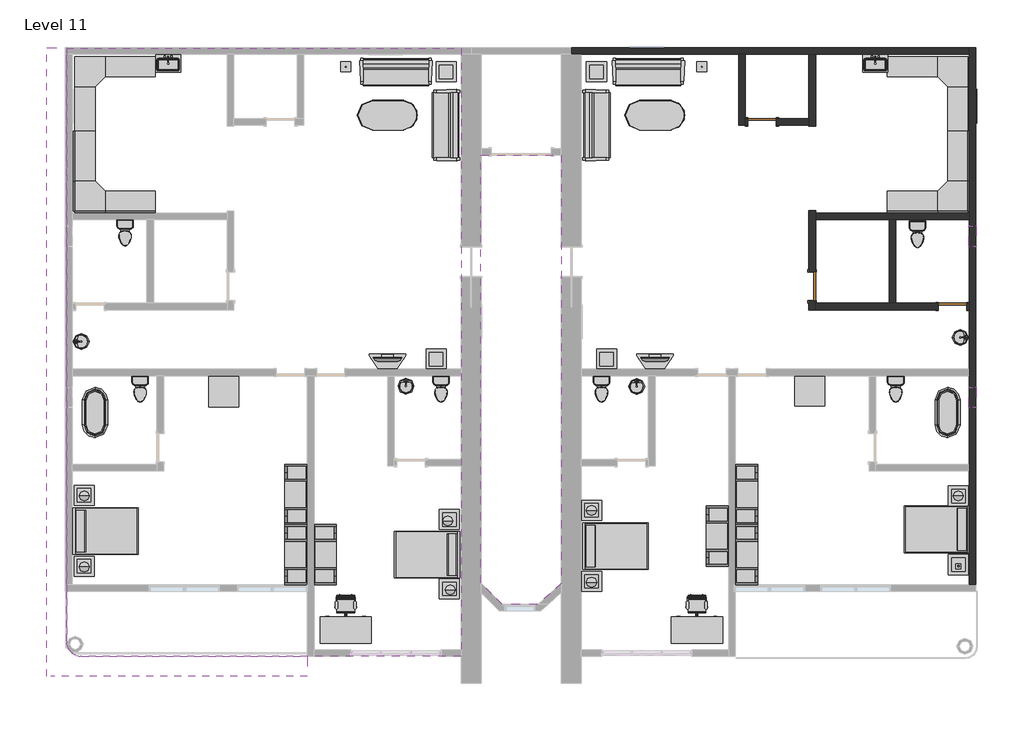
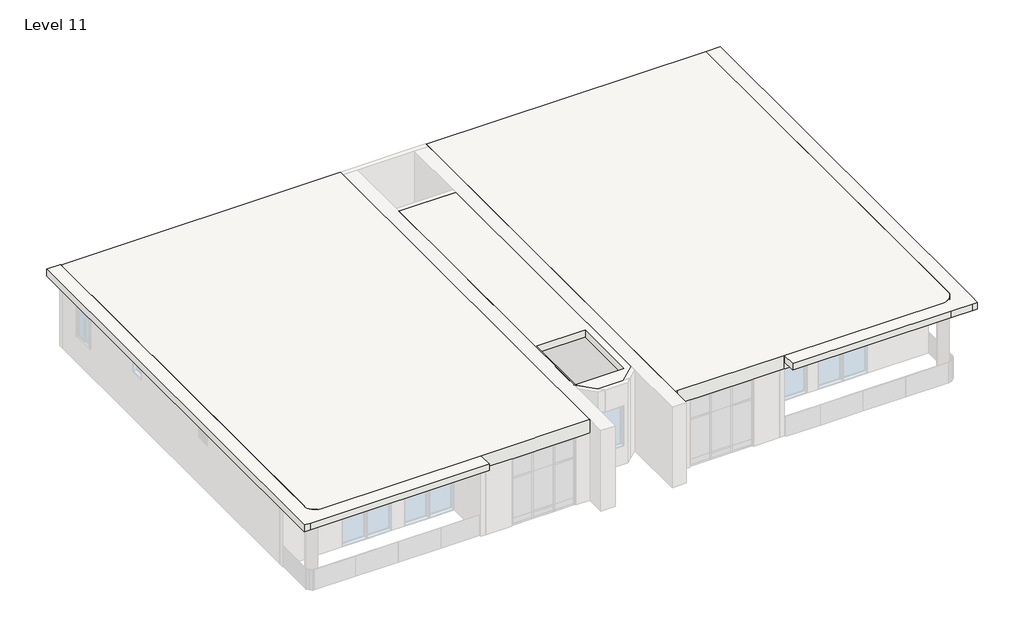
# One storey, part 3 of 3: 42 furniture elements, 14 flow terminals, 10 light fixtures, 9 walls, 3 doors, 3 slabs, 3 windows.
"""IFC4 building model written with IfcOpenShell, lengths in millimetres."""

from ifc_helpers import new_model, si_unit, point, frame, frame_2d, origin, place, context, project, spatial, polyline, circle_curve, trimmed, segment, composite_curve, outline, extrude, faceted_brep, transform, mapped, element, save
from components import door_2703ae13, door_10fd3a06, flow_terminal_38af2918, flow_terminal_d49f872f, toilet_domestic_3d_toilet_domestic_3d_f7549cf7, toilet_domestic_3d_toilet_domestic_3d_183bbd19, flow_terminal_b374fae2, furniture_07436f11, furniture_096e7f55, chair_task_arms_chair_task_arms_fa5a08ef, furniture_072f6425, furniture_cf0b6580, furniture_aff9b2fb, furniture_56245f3a, tv_stand_tv_stand_6ce107e5, furniture_b5c51a22, furniture_2c34a4f9, furniture_4d44e21c, furniture_45e3acac, light_fixture_100w_120v_8564026f, table_lamp_hemispheric_60w_120v_02721d88, window_0038ecf3, window_54100e87

model = new_model("IFC4")

# Units and contexts
model_context = context("Model", 3, world=origin())
ifc_project = project(units=[si_unit("LENGTHUNIT", "METRE", prefix="MILLI")], contexts=[model_context])

# Site, building, storey
site = spatial("IfcSite", under=ifc_project)
building = spatial("IfcBuilding", under=site)
storey = spatial("IfcBuildingStorey", under=building, Name="Level 11", Elevation=36576.0)

# Doors
placement = place(None, origin())
door_shape = door_2703ae13(model_context)
element("IfcDoor", 1, ObjectType="Door-Single-Panel.0001 : 34\" x 80\"", at=placement, inside=storey, context=model_context, shape_type="MappedRepresentation", body=[
    mapped(door_shape, transform((2528.3512296, 9464.0758558, 36576.0), x_axis=(-1.0, 0.0, 0.0), y_axis=(0.0, -1.0, 0.0), z_axis=(0.0, 0.0, 1.0))),
])
door_2_shape = door_10fd3a06(model_context)
element("IfcDoor", 2, ObjectType="Door-Single-Panel.0001 : 34\" x 80\"", at=placement, inside=storey, context=model_context, shape_type="MappedRepresentation", body=[
    mapped(door_2_shape, transform((8319.5512296, 3850.6758558, 36576.0), x_axis=(1.0, 0.0, 0.0), y_axis=(0.0, 1.0, 0.0), z_axis=(0.0, 0.0, 1.0))),
])
element("IfcDoor", 3, ObjectType="Door-Single-Panel.0001 : 34\" x 80\"", at=placement, inside=storey, context=model_context, shape_type="MappedRepresentation", body=[
    mapped(door_2_shape, transform((4052.3512296, 4460.2758558, 36576.0), x_axis=(0.0, -1.0, 0.0), y_axis=(1.0, 0.0, 0.0), z_axis=(0.0, 0.0, 1.0))),
])

# Flow terminals
flow_terminal_shape = flow_terminal_38af2918(model_context)
element("IfcFlowTerminal", 4, ObjectType="Sink Kitchen-Single : 30\" x 21\"", at=placement, inside=storey, context=model_context, shape_type="MappedRepresentation", body=[
    mapped(flow_terminal_shape, transform((-15534.038011, 11239.7304546, 36576.0), x_axis=(1.0, 0.0, 0.0), y_axis=(0.0, 1.0, 0.0), z_axis=(0.0, 0.0, 1.0))),
])
element("IfcFlowTerminal", 5, ObjectType="Sink Kitchen-Single : 30\" x 21\"", at=placement, inside=storey, context=model_context, shape_type="MappedRepresentation", body=[
    mapped(flow_terminal_shape, transform((5954.361989, 11239.7304546, 36576.0), x_axis=(1.0, 0.0, 0.0), y_axis=(0.0, 1.0, 0.0), z_axis=(0.0, 0.0, 1.0))),
])
flow_terminal_2_shape = flow_terminal_d49f872f(model_context)
element("IfcFlowTerminal", 6, ObjectType="Sink Vanity-Round : 19\" x 19\"", at=placement, inside=storey, context=model_context, shape_type="MappedRepresentation", body=[
    mapped(flow_terminal_2_shape, transform((-18078.2570794, 2687.2241152, 36576.0), x_axis=(0.0, 1.0, 0.0), y_axis=(-1.0, 0.0, 0.0), z_axis=(0.0, 0.0, 1.0))),
])
element("IfcFlowTerminal", 7, ObjectType="Sink Vanity-Round : 19\" x 19\"", at=placement, inside=storey, context=model_context, shape_type="MappedRepresentation", body=[
    mapped(flow_terminal_2_shape, transform((8468.5749463, 3007.5275963, 36576.0), x_axis=(0.0, -1.0, 0.0), y_axis=(1.0, 0.0, 0.0), z_axis=(0.0, 0.0, 1.0))),
])
element("IfcFlowTerminal", 8, ObjectType="Sink Vanity-Round : 19\" x 19\"", at=placement, inside=storey, context=model_context, shape_type="MappedRepresentation", body=[
    mapped(flow_terminal_2_shape, transform((-8388.700511, 1341.8921141, 36576.0), x_axis=(1.0, 0.0, 0.0), y_axis=(0.0, 1.0, 0.0), z_axis=(0.0, 0.0, 1.0))),
])
element("IfcFlowTerminal", 9, ObjectType="Sink Vanity-Round : 19\" x 19\"", at=placement, inside=storey, context=model_context, shape_type="MappedRepresentation", body=[
    mapped(flow_terminal_2_shape, transform((-1378.300511, 1331.0855344, 36576.0), x_axis=(1.0, 0.0, 0.0), y_axis=(0.0, 1.0, 0.0), z_axis=(0.0, 0.0, 1.0))),
])
toilet_domestic_3d_toilet_domestic_3d_shape = toilet_domestic_3d_toilet_domestic_3d_f7549cf7(model_context)
toilet_domestic_3d_toilet_domestic_3d_2_shape = toilet_domestic_3d_toilet_domestic_3d_183bbd19(model_context)
element("IfcFlowTerminal", 10, ObjectType="Toilet-Domestic-3D : Toilet-Domestic-3D", at=placement, inside=storey, context=model_context, shape_type="MappedRepresentation", body=[
    mapped(toilet_domestic_3d_toilet_domestic_3d_shape, transform((6592.3512296, 1247.7798284, 36576.0), x_axis=(1.0, 0.0, 0.0), y_axis=(0.0, 1.0, 0.0), z_axis=(0.0, 0.0, 1.0))),
    mapped(toilet_domestic_3d_toilet_domestic_3d_2_shape, transform((6592.3512296, 1247.7798284, 36576.0), x_axis=(1.0, 0.0, 0.0), y_axis=(0.0, 1.0, 0.0), z_axis=(0.0, 0.0, 1.0))),
])
element("IfcFlowTerminal", 11, ObjectType="Toilet-Domestic-3D : Toilet-Domestic-3D", at=placement, inside=storey, context=model_context, shape_type="MappedRepresentation", body=[
    mapped(toilet_domestic_3d_toilet_domestic_3d_shape, transform((-2348.4487704, 1247.7798284, 36576.0), x_axis=(1.0, 0.0, 0.0), y_axis=(0.0, 1.0, 0.0), z_axis=(0.0, 0.0, 1.0))),
    mapped(toilet_domestic_3d_toilet_domestic_3d_2_shape, transform((-2348.4487704, 1247.7798284, 36576.0), x_axis=(1.0, 0.0, 0.0), y_axis=(0.0, 1.0, 0.0), z_axis=(0.0, 0.0, 1.0))),
])
element("IfcFlowTerminal", 12, ObjectType="Toilet-Domestic-3D : Toilet-Domestic-3D", at=placement, inside=storey, context=model_context, shape_type="MappedRepresentation", body=[
    mapped(toilet_domestic_3d_toilet_domestic_3d_shape, transform((-16369.2487704, 1247.7798284, 36576.0), x_axis=(1.0, 0.0, 0.0), y_axis=(0.0, 1.0, 0.0), z_axis=(0.0, 0.0, 1.0))),
    mapped(toilet_domestic_3d_toilet_domestic_3d_2_shape, transform((-16369.2487704, 1247.7798284, 36576.0), x_axis=(1.0, 0.0, 0.0), y_axis=(0.0, 1.0, 0.0), z_axis=(0.0, 0.0, 1.0))),
])
element("IfcFlowTerminal", 13, ObjectType="Toilet-Domestic-3D : Toilet-Domestic-3D", at=placement, inside=storey, context=model_context, shape_type="MappedRepresentation", body=[
    mapped(toilet_domestic_3d_toilet_domestic_3d_shape, transform((-16826.4487704, 5997.5798284, 36576.0), x_axis=(1.0, 0.0, 0.0), y_axis=(0.0, 1.0, 0.0), z_axis=(0.0, 0.0, 1.0))),
    mapped(toilet_domestic_3d_toilet_domestic_3d_2_shape, transform((-16826.4487704, 5997.5798284, 36576.0), x_axis=(1.0, 0.0, 0.0), y_axis=(0.0, 1.0, 0.0), z_axis=(0.0, 0.0, 1.0))),
])
element("IfcFlowTerminal", 14, ObjectType="Toilet-Domestic-3D : Toilet-Domestic-3D", at=placement, inside=storey, context=model_context, shape_type="MappedRepresentation", body=[
    mapped(toilet_domestic_3d_toilet_domestic_3d_shape, transform((7252.7512296, 5946.7798284, 36576.0), x_axis=(1.0, 0.0, 0.0), y_axis=(0.0, 1.0, 0.0), z_axis=(0.0, 0.0, 1.0))),
    mapped(toilet_domestic_3d_toilet_domestic_3d_2_shape, transform((7252.7512296, 5946.7798284, 36576.0), x_axis=(1.0, 0.0, 0.0), y_axis=(0.0, 1.0, 0.0), z_axis=(0.0, 0.0, 1.0))),
])
element("IfcFlowTerminal", 15, ObjectType="Toilet-Domestic-3D : Toilet-Domestic-3D", at=placement, inside=storey, context=model_context, shape_type="MappedRepresentation", body=[
    mapped(toilet_domestic_3d_toilet_domestic_3d_shape, transform((-7225.2487704, 1247.7798284, 36576.0), x_axis=(1.0, 0.0, 0.0), y_axis=(0.0, 1.0, 0.0), z_axis=(0.0, 0.0, 1.0))),
    mapped(toilet_domestic_3d_toilet_domestic_3d_2_shape, transform((-7225.2487704, 1247.7798284, 36576.0), x_axis=(1.0, 0.0, 0.0), y_axis=(0.0, 1.0, 0.0), z_axis=(0.0, 0.0, 1.0))),
])
flow_terminal_3_shape = flow_terminal_b374fae2(model_context)
element("IfcFlowTerminal", 16, ObjectType="Tub-Free Standing-3D : 30\" x 60\"", at=placement, inside=storey, context=model_context, shape_type="MappedRepresentation", body=[
    mapped(flow_terminal_3_shape, transform((-17740.8487704, 624.8758558, 36576.0), x_axis=(1.0, 0.0, 0.0), y_axis=(0.0, 1.0, 0.0), z_axis=(0.0, 0.0, 1.0))),
])
element("IfcFlowTerminal", 17, ObjectType="Tub-Free Standing-3D : 30\" x 60\"", at=placement, inside=storey, context=model_context, shape_type="MappedRepresentation", body=[
    mapped(flow_terminal_3_shape, transform((8167.1512296, 624.8758558, 36576.0), x_axis=(1.0, 0.0, 0.0), y_axis=(0.0, 1.0, 0.0), z_axis=(0.0, 0.0, 1.0))),
])

# Furniture
furniture_shape = furniture_07436f11(model_context)
element("IfcFurniture", 18, ObjectType="96\" x 96\"", at=placement, inside=storey, context=model_context, shape_type="MappedRepresentation", body=[
    mapped(furniture_shape, transform((-18269.5170182, 11991.0988634, 36576.0), x_axis=(1.0, 0.0, 0.0), y_axis=(0.0, 1.0, 0.0), z_axis=(0.0, 0.0, 1.0))),
])
element("IfcFurniture", 19, ObjectType="96\" x 96\"", at=placement, inside=storey, context=model_context, shape_type="MappedRepresentation", body=[
    mapped(furniture_shape, transform((9322.5742372, 11364.3441035, 36576.0), x_axis=(0.0, -1.0, 0.0), y_axis=(1.0, 0.0, 0.0), z_axis=(0.0, 0.0, 1.0))),
])
furniture_2_shape = furniture_096e7f55(model_context)
element("IfcFurniture", 20, ObjectType="Bed-Shaker : Double 56\" x 78\"", at=placement, inside=storey, context=model_context, shape_type="MappedRepresentation", body=[
    mapped(furniture_2_shape, transform((-18401.2487704, -2962.8741442, 36576.0), x_axis=(0.0, 1.0, 0.0), y_axis=(-1.0, 0.0, 0.0), z_axis=(0.0, 0.0, 1.0))),
])
element("IfcFurniture", 21, ObjectType="Bed-Shaker : Double 56\" x 78\"", at=placement, inside=storey, context=model_context, shape_type="MappedRepresentation", body=[
    mapped(furniture_2_shape, transform((-6666.4487704, -3712.1741442, 36576.0), x_axis=(0.0, -1.0, 0.0), y_axis=(1.0, 0.0, 0.0), z_axis=(0.0, 0.0, 1.0))),
])
element("IfcFurniture", 22, ObjectType="Bed-Shaker : Double 56\" x 78\"", at=placement, inside=storey, context=model_context, shape_type="MappedRepresentation", body=[
    mapped(furniture_2_shape, transform((-2907.2487704, -3420.0741442, 36576.0), x_axis=(0.0, 1.0, 0.0), y_axis=(-1.0, 0.0, 0.0), z_axis=(0.0, 0.0, 1.0))),
])
element("IfcFurniture", 23, ObjectType="Bed-Shaker : Double 56\" x 78\"", at=placement, inside=storey, context=model_context, shape_type="MappedRepresentation", body=[
    mapped(furniture_2_shape, transform((8827.5512296, -2950.1741442, 36576.0), x_axis=(0.0, -1.0, 0.0), y_axis=(1.0, 0.0, 0.0), z_axis=(0.0, 0.0, 1.0))),
])
chair_task_arms_chair_task_arms_shape = chair_task_arms_chair_task_arms_fa5a08ef(model_context)
element("IfcFurniture", 24, ObjectType="Chair-Task Arms : Chair-Task Arms", at=placement, inside=storey, context=model_context, shape_type="MappedRepresentation", body=[
    mapped(chair_task_arms_chair_task_arms_shape, transform((688.1420493, -5184.3566833, 36576.0), x_axis=(-1.0, 0.0, 0.0), y_axis=(0.0, -1.0, 0.0), z_axis=(0.0, 0.0, 1.0))),
])
element("IfcFurniture", 25, ObjectType="Chair-Task Arms : Chair-Task Arms", at=placement, inside=storey, context=model_context, shape_type="MappedRepresentation", body=[
    mapped(chair_task_arms_chair_task_arms_shape, transform((-9979.8579507, -5184.3566833, 36576.0), x_axis=(-1.0, 0.0, 0.0), y_axis=(0.0, -1.0, 0.0), z_axis=(0.0, 0.0, 1.0))),
])
furniture_3_shape = furniture_072f6425(model_context)
element("IfcFurniture", 26, ObjectType="Desk : 60\" x 30\"", at=placement, inside=storey, context=model_context, shape_type="MappedRepresentation", body=[
    mapped(furniture_3_shape, transform((-10882.8487704, -6371.702585, 36576.0), x_axis=(1.0, 0.0, 0.0), y_axis=(0.0, 1.0, 0.0), z_axis=(0.0, 0.0, 1.0))),
])
element("IfcFurniture", 27, ObjectType="Desk : 60\" x 30\"", at=placement, inside=storey, context=model_context, shape_type="MappedRepresentation", body=[
    mapped(furniture_3_shape, transform((-214.8487704, -6371.702585, 36576.0), x_axis=(1.0, 0.0, 0.0), y_axis=(0.0, 1.0, 0.0), z_axis=(0.0, 0.0, 1.0))),
])
furniture_4_shape = furniture_cf0b6580(model_context)
element("IfcFurniture", 28, ObjectType="Entertainment Center : 72\" x 72\" x 24\"", at=placement, inside=storey, context=model_context, shape_type="MappedRepresentation", body=[
    mapped(furniture_4_shape, transform((1613.9512296, -3134.3241442, 36576.0), x_axis=(0.0, -1.0, 0.0), y_axis=(1.0, 0.0, 0.0), z_axis=(0.0, 0.0, 1.0))),
])
element("IfcFurniture", 29, ObjectType="Entertainment Center : 72\" x 72\" x 24\"", at=placement, inside=storey, context=model_context, shape_type="MappedRepresentation", body=[
    mapped(furniture_4_shape, transform((1613.9512296, -3693.1241442, 36576.0), x_axis=(0.0, 1.0, 0.0), y_axis=(-1.0, 0.0, 0.0), z_axis=(0.0, 0.0, 1.0))),
])
element("IfcFurniture", 30, ObjectType="Entertainment Center : 72\" x 72\" x 24\"", at=placement, inside=storey, context=model_context, shape_type="MappedRepresentation", body=[
    mapped(furniture_4_shape, transform((1613.9512296, -1864.3241442, 36576.0), x_axis=(0.0, 1.0, 0.0), y_axis=(-1.0, 0.0, 0.0), z_axis=(0.0, 0.0, 1.0))),
])
element("IfcFurniture", 31, ObjectType="Entertainment Center : 72\" x 72\" x 24\"", at=placement, inside=storey, context=model_context, shape_type="MappedRepresentation", body=[
    mapped(furniture_4_shape, transform((-11187.6487704, -3693.1241442, 36576.0), x_axis=(0.0, -1.0, 0.0), y_axis=(1.0, 0.0, 0.0), z_axis=(0.0, 0.0, 1.0))),
])
element("IfcFurniture", 32, ObjectType="Entertainment Center : 72\" x 72\" x 24\"", at=placement, inside=storey, context=model_context, shape_type="MappedRepresentation", body=[
    mapped(furniture_4_shape, transform((-11187.6487704, -1864.3241442, 36576.0), x_axis=(0.0, -1.0, 0.0), y_axis=(1.0, 0.0, 0.0), z_axis=(0.0, 0.0, 1.0))),
])
element("IfcFurniture", 33, ObjectType="Entertainment Center : 72\" x 72\" x 24\"", at=placement, inside=storey, context=model_context, shape_type="MappedRepresentation", body=[
    mapped(furniture_4_shape, transform((-11187.6487704, -3693.1241442, 36576.0), x_axis=(0.0, 1.0, 0.0), y_axis=(-1.0, 0.0, 0.0), z_axis=(0.0, 0.0, 1.0))),
])
furniture_5_shape = furniture_aff9b2fb(model_context)
element("IfcFurniture", 34, ObjectType="Sofa-Pensi : 84\"", at=placement, inside=storey, context=model_context, shape_type="MappedRepresentation", body=[
    mapped(furniture_5_shape, transform((-8875.4550204, 10710.9660197, 36576.0), x_axis=(1.0, 0.0, 0.0), y_axis=(0.0, 1.0, 0.0), z_axis=(0.0, 0.0, 1.0))),
])
element("IfcFurniture", 35, ObjectType="Sofa-Pensi : 84\"", at=placement, inside=storey, context=model_context, shape_type="MappedRepresentation", body=[
    mapped(furniture_5_shape, transform((-7349.9586065, 9641.0821058, 36576.0), x_axis=(0.0, -1.0, 0.0), y_axis=(1.0, 0.0, 0.0), z_axis=(0.0, 0.0, 1.0))),
])
element("IfcFurniture", 36, ObjectType="Sofa-Pensi : 84\"", at=placement, inside=storey, context=model_context, shape_type="MappedRepresentation", body=[
    mapped(furniture_5_shape, transform((-2223.7389343, 9083.8696058, 36576.0), x_axis=(0.0, 1.0, 0.0), y_axis=(-1.0, 0.0, 0.0), z_axis=(0.0, 0.0, 1.0))),
])
element("IfcFurniture", 37, ObjectType="Sofa-Pensi : 84\"", at=placement, inside=storey, context=model_context, shape_type="MappedRepresentation", body=[
    mapped(furniture_5_shape, transform((-1204.6550204, 10710.9660197, 36576.0), x_axis=(1.0, 0.0, 0.0), y_axis=(0.0, 1.0, 0.0), z_axis=(0.0, 0.0, 1.0))),
])
furniture_6_shape = furniture_56245f3a(model_context)
element("IfcFurniture", 38, ObjectType="TV - Flat Screen : 32\"", at=placement, inside=storey, context=model_context, shape_type="MappedRepresentation", body=[
    mapped(furniture_6_shape, transform((-8854.7932846, 2232.8144794, 37490.4), x_axis=(-1.0, 0.0, 0.0), y_axis=(0.0, -1.0, 0.0), z_axis=(0.0, 0.0, 1.0))),
])
element("IfcFurniture", 39, ObjectType="TV - Flat Screen : 32\"", at=placement, inside=storey, context=model_context, shape_type="MappedRepresentation", body=[
    mapped(furniture_6_shape, transform((-726.7932846, 2232.8144794, 37490.4), x_axis=(-1.0, 0.0, 0.0), y_axis=(0.0, -1.0, 0.0), z_axis=(0.0, 0.0, 1.0))),
])
tv_stand_tv_stand_shape = tv_stand_tv_stand_6ce107e5(model_context)
element("IfcFurniture", 40, ObjectType="TV Stand : TV Stand", at=placement, inside=storey, context=model_context, shape_type="MappedRepresentation", body=[
    mapped(tv_stand_tv_stand_shape, transform((-8725.6607683, 1945.6758558, 36576.0), x_axis=(-1.0, 0.0, 0.0), y_axis=(0.0, -1.0, 0.0), z_axis=(0.0, 0.0, 1.0))),
])
element("IfcFurniture", 41, ObjectType="TV Stand : TV Stand", at=placement, inside=storey, context=model_context, shape_type="MappedRepresentation", body=[
    mapped(tv_stand_tv_stand_shape, transform((-597.6607683, 1945.6758558, 36576.0), x_axis=(-1.0, 0.0, 0.0), y_axis=(0.0, -1.0, 0.0), z_axis=(0.0, 0.0, 1.0))),
])
furniture_7_shape = furniture_b5c51a22(model_context)
element("IfcFurniture", 42, ObjectType="Table-Coffee : 24\" x 24\" x 24\"", at=placement, inside=storey, context=model_context, shape_type="MappedRepresentation", body=[
    mapped(furniture_7_shape, transform((-7091.1145371, 10892.864778, 36576.0), x_axis=(1.0, 0.0, 0.0), y_axis=(0.0, 1.0, 0.0), z_axis=(0.0, 0.0, 1.0))),
])
element("IfcFurniture", 43, ObjectType="Table-Coffee : 24\" x 24\" x 24\"", at=placement, inside=storey, context=model_context, shape_type="MappedRepresentation", body=[
    mapped(furniture_7_shape, transform((-2519.1145371, 10892.864778, 36576.0), x_axis=(1.0, 0.0, 0.0), y_axis=(0.0, 1.0, 0.0), z_axis=(0.0, 0.0, 1.0))),
])
element("IfcFurniture", 44, ObjectType="Table-Coffee : 24\" x 24\" x 24\"", at=placement, inside=storey, context=model_context, shape_type="MappedRepresentation", body=[
    mapped(furniture_7_shape, transform((-7395.9145371, 2155.264778, 36576.0), x_axis=(1.0, 0.0, 0.0), y_axis=(0.0, 1.0, 0.0), z_axis=(0.0, 0.0, 1.0))),
])
element("IfcFurniture", 45, ObjectType="Table-Coffee : 24\" x 24\" x 24\"", at=placement, inside=storey, context=model_context, shape_type="MappedRepresentation", body=[
    mapped(furniture_7_shape, transform((-2214.3145371, 2155.264778, 36576.0), x_axis=(1.0, 0.0, 0.0), y_axis=(0.0, 1.0, 0.0), z_axis=(0.0, 0.0, 1.0))),
])
element("IfcFurniture", 46, ObjectType="Table-Coffee : 24\" x 24\" x 24\"", at=placement, inside=storey, context=model_context, shape_type="MappedRepresentation", body=[
    mapped(furniture_7_shape, transform((-2671.5145371, -4601.135222, 36576.0), x_axis=(1.0, 0.0, 0.0), y_axis=(0.0, 1.0, 0.0), z_axis=(0.0, 0.0, 1.0))),
])
element("IfcFurniture", 47, ObjectType="Table-Coffee : 24\" x 24\" x 24\"", at=placement, inside=storey, context=model_context, shape_type="MappedRepresentation", body=[
    mapped(furniture_7_shape, transform((-18089.3145371, -4143.935222, 36576.0), x_axis=(1.0, 0.0, 0.0), y_axis=(0.0, 1.0, 0.0), z_axis=(0.0, 0.0, 1.0))),
])
element("IfcFurniture", 48, ObjectType="Table-Coffee : 24\" x 24\" x 24\"", at=placement, inside=storey, context=model_context, shape_type="MappedRepresentation", body=[
    mapped(furniture_7_shape, transform((-18089.3145371, -1984.935222, 36576.0), x_axis=(1.0, 0.0, 0.0), y_axis=(0.0, 1.0, 0.0), z_axis=(0.0, 0.0, 1.0))),
])
element("IfcFurniture", 49, ObjectType="Table-Coffee : 24\" x 24\" x 24\"", at=placement, inside=storey, context=model_context, shape_type="MappedRepresentation", body=[
    mapped(furniture_7_shape, transform((-2671.5145371, -2442.135222, 36576.0), x_axis=(1.0, 0.0, 0.0), y_axis=(0.0, 1.0, 0.0), z_axis=(0.0, 0.0, 1.0))),
])
element("IfcFurniture", 50, ObjectType="Table-Coffee : 24\" x 24\" x 24\"", at=placement, inside=storey, context=model_context, shape_type="MappedRepresentation", body=[
    mapped(furniture_7_shape, transform((8479.0854629, -4093.135222, 36576.0), x_axis=(1.0, 0.0, 0.0), y_axis=(0.0, 1.0, 0.0), z_axis=(0.0, 0.0, 1.0))),
])
element("IfcFurniture", 51, ObjectType="Table-Coffee : 24\" x 24\" x 24\"", at=placement, inside=storey, context=model_context, shape_type="MappedRepresentation", body=[
    mapped(furniture_7_shape, transform((8479.0854629, -2010.335222, 36576.0), x_axis=(1.0, 0.0, 0.0), y_axis=(0.0, 1.0, 0.0), z_axis=(0.0, 0.0, 1.0))),
])
element("IfcFurniture", 52, ObjectType="Table-Coffee : 24\" x 24\" x 24\"", at=placement, inside=storey, context=model_context, shape_type="MappedRepresentation", body=[
    mapped(furniture_7_shape, transform((-6989.5145371, -4832.0414601, 36576.0), x_axis=(1.0, 0.0, 0.0), y_axis=(0.0, 1.0, 0.0), z_axis=(0.0, 0.0, 1.0))),
])
element("IfcFurniture", 53, ObjectType="Table-Coffee : 24\" x 24\" x 24\"", at=placement, inside=storey, context=model_context, shape_type="MappedRepresentation", body=[
    mapped(furniture_7_shape, transform((-6989.5145371, -2723.8414601, 36576.0), x_axis=(1.0, 0.0, 0.0), y_axis=(0.0, 1.0, 0.0), z_axis=(0.0, 0.0, 1.0))),
])
furniture_8_shape = furniture_2c34a4f9(model_context)
element("IfcFurniture", 54, ObjectType="Table-Dining Oval : 36\" x 72\"", at=placement, inside=storey, context=model_context, shape_type="MappedRepresentation", body=[
    mapped(furniture_8_shape, transform((-8449.0290983, 10025.3742164, 36576.0), x_axis=(1.0, 0.0, 0.0), y_axis=(0.0, 1.0, 0.0), z_axis=(0.0, 0.0, 1.0))),
])
element("IfcFurniture", 55, ObjectType="Table-Dining Oval : 36\" x 72\"", at=placement, inside=storey, context=model_context, shape_type="MappedRepresentation", body=[
    mapped(furniture_8_shape, transform((-321.0290983, 10025.3742164, 36576.0), x_axis=(1.0, 0.0, 0.0), y_axis=(0.0, 1.0, 0.0), z_axis=(0.0, 0.0, 1.0))),
])
furniture_9_shape = furniture_4d44e21c(model_context)
element("IfcFurniture", 56, ObjectType="Table-Rectangular : 36\" x 36\"", at=placement, inside=storey, context=model_context, shape_type="MappedRepresentation", body=[
    mapped(furniture_9_shape, transform((-13829.2487704, 1259.8758558, 36576.0), x_axis=(1.0, 0.0, 0.0), y_axis=(0.0, 1.0, 0.0), z_axis=(0.0, 0.0, 1.0))),
])
element("IfcFurniture", 57, ObjectType="Table-Rectangular : 36\" x 36\"", at=placement, inside=storey, context=model_context, shape_type="MappedRepresentation", body=[
    mapped(furniture_9_shape, transform((3976.1512296, 1285.2758558, 36576.0), x_axis=(1.0, 0.0, 0.0), y_axis=(0.0, 1.0, 0.0), z_axis=(0.0, 0.0, 1.0))),
])
furniture_10_shape = furniture_45e3acac(model_context)
element("IfcFurniture", 58, ObjectType="Work Station Cubicle : 96\" x 96\"", at=placement, inside=storey, context=model_context, shape_type="MappedRepresentation", body=[
    mapped(furniture_10_shape, transform((-18896.271778, 6827.207608, 36576.0), x_axis=(0.0, 1.0, 0.0), y_axis=(-1.0, 0.0, 0.0), z_axis=(0.0, 0.0, 1.0))),
])
element("IfcFurniture", 59, ObjectType="Work Station Cubicle : 96\" x 96\"", at=placement, inside=storey, context=model_context, shape_type="MappedRepresentation", body=[
    mapped(furniture_10_shape, transform((8695.8194774, 6200.4528481, 36576.0), x_axis=(-1.0, 0.0, 0.0), y_axis=(0.0, -1.0, 0.0), z_axis=(0.0, 0.0, 1.0))),
])

# Light fixtures
light_fixture_100w_120v_shape = light_fixture_100w_120v_8564026f(model_context)
element("IfcLightFixture", 60, ObjectType="100W - 120V", at=placement, inside=storey, context=model_context, shape_type="MappedRepresentation", body=[
    mapped(light_fixture_100w_120v_shape, transform((-10120.8487704, 11140.4758558, 36576.0), x_axis=(1.0, 0.0, 0.0), y_axis=(0.0, 1.0, 0.0), z_axis=(0.0, 0.0, 1.0))),
])
element("IfcLightFixture", 61, ObjectType="100W - 120V", at=placement, inside=storey, context=model_context, shape_type="MappedRepresentation", body=[
    mapped(light_fixture_100w_120v_shape, transform((699.5512296, 11140.4758558, 36576.0), x_axis=(1.0, 0.0, 0.0), y_axis=(0.0, 1.0, 0.0), z_axis=(0.0, 0.0, 1.0))),
])
table_lamp_hemispheric_60w_120v_shape = table_lamp_hemispheric_60w_120v_02721d88(model_context)
element("IfcLightFixture", 62, ObjectType="Table Lamp - Hemispheric : 60W - 120V", at=placement, inside=storey, context=model_context, shape_type="MappedRepresentation", body=[
    mapped(table_lamp_hemispheric_60w_120v_shape, transform((-18071.0487704, -1915.1241442, 37185.6), x_axis=(1.0, 0.0, 0.0), y_axis=(0.0, 1.0, 0.0), z_axis=(0.0, 0.0, 1.0))),
])
element("IfcLightFixture", 63, ObjectType="Table Lamp - Hemispheric : 60W - 120V", at=placement, inside=storey, context=model_context, shape_type="MappedRepresentation", body=[
    mapped(table_lamp_hemispheric_60w_120v_shape, transform((-7022.0487704, -2666.7303823, 37185.6), x_axis=(1.0, 0.0, 0.0), y_axis=(0.0, 1.0, 0.0), z_axis=(0.0, 0.0, 1.0))),
])
element("IfcLightFixture", 64, ObjectType="Table Lamp - Hemispheric : 60W - 120V", at=placement, inside=storey, context=model_context, shape_type="MappedRepresentation", body=[
    mapped(table_lamp_hemispheric_60w_120v_shape, transform((-2653.2487704, -2346.9241442, 37185.6), x_axis=(1.0, 0.0, 0.0), y_axis=(0.0, 1.0, 0.0), z_axis=(0.0, 0.0, 1.0))),
])
element("IfcLightFixture", 65, ObjectType="Table Lamp - Hemispheric : 60W - 120V", at=placement, inside=storey, context=model_context, shape_type="MappedRepresentation", body=[
    mapped(table_lamp_hemispheric_60w_120v_shape, transform((8497.3512296, -4048.7241442, 37490.4), x_axis=(1.0, 0.0, 0.0), y_axis=(0.0, 1.0, 0.0), z_axis=(0.0, 0.0, 1.0))),
])
element("IfcLightFixture", 66, ObjectType="Table Lamp - Hemispheric : 60W - 120V", at=placement, inside=storey, context=model_context, shape_type="MappedRepresentation", body=[
    mapped(table_lamp_hemispheric_60w_120v_shape, transform((8497.3512296, -1915.1241442, 37185.6), x_axis=(1.0, 0.0, 0.0), y_axis=(0.0, 1.0, 0.0), z_axis=(0.0, 0.0, 1.0))),
])
element("IfcLightFixture", 67, ObjectType="Table Lamp - Hemispheric : 60W - 120V", at=placement, inside=storey, context=model_context, shape_type="MappedRepresentation", body=[
    mapped(table_lamp_hemispheric_60w_120v_shape, transform((-2653.2487704, -4531.3241442, 37185.6), x_axis=(1.0, 0.0, 0.0), y_axis=(0.0, 1.0, 0.0), z_axis=(0.0, 0.0, 1.0))),
])
element("IfcLightFixture", 68, ObjectType="Table Lamp - Hemispheric : 60W - 120V", at=placement, inside=storey, context=model_context, shape_type="MappedRepresentation", body=[
    mapped(table_lamp_hemispheric_60w_120v_shape, transform((-6945.8487704, -4762.2303823, 37185.6), x_axis=(1.0, 0.0, 0.0), y_axis=(0.0, 1.0, 0.0), z_axis=(0.0, 0.0, 1.0))),
])
element("IfcLightFixture", 69, ObjectType="Table Lamp - Hemispheric : 60W - 120V", at=placement, inside=storey, context=model_context, shape_type="MappedRepresentation", body=[
    mapped(table_lamp_hemispheric_60w_120v_shape, transform((-18071.0487704, -4074.1241442, 37185.6), x_axis=(1.0, 0.0, 0.0), y_axis=(0.0, 1.0, 0.0), z_axis=(0.0, 0.0, 1.0))),
])

# Slabs
element("IfcSlab", 70, ObjectType="Generic - 12\" cream", at=placement, inside=storey, context=model_context, shape_type="SweptSolid", body=[
    extrude(outline(composite_curve([segment(polyline([(-6615.6487704, 11699.2758558), (-6615.6487704, -6791.9241442), (-11289.2487704, -6791.9241442), (-18147.2487704, -6791.9241442)]), True, "CONTINUOUS"), segment(trimmed(circle_curve(frame_2d((-18147.2487704, -6334.7241442)), 457.2), [point((-18147.2487704, -6791.9241442))], [point((-18604.4487704, -6334.7241442))], False, "CARTESIAN"), True, "CONTINUOUS"), segment(polyline([(-18604.4487704, -6334.7241442), (-18604.4487704, 11699.2758558), (-6615.6487704, 11699.2758558)]), True, "CONTINUOUS")], self_intersect=False)), frame((0.0, 0.0, 39624.0), z_axis=(0.0, 0.0, 1.0), x_axis=(1.0, 0.0, 0.0)), (0.0, 0.0, 1.0), 609.6),
    extrude(outline(composite_curve([segment(trimmed(circle_curve(frame_2d((8518.1543381, -6277.3874522)), 514.536692), [point((9030.7512296, -6322.0241442))], [point((8518.1543381, -6791.9241442))], False, "CARTESIAN"), True, "CONTINUOUS"), segment(polyline([(8518.1543381, -6791.9241442), (1715.5512296, -6791.9241442), (-2856.4487704, -6791.9241442), (-2958.0487704, -6791.9241442), (-2958.0487704, 11699.2758558), (9030.7512296, 11699.2758558), (9030.7512296, -6322.0241442)]), True, "CONTINUOUS")], self_intersect=False)), frame((0.0, 0.0, 39624.0), z_axis=(0.0, 0.0, 1.0), x_axis=(1.0, 0.0, 0.0)), (0.0, 0.0, 1.0), 609.6),
])
element("IfcSlab", 71, ObjectType="Generic - 12\" white", at=placement, inside=storey, context=model_context, shape_type="SweptSolid", body=[
    extrude(outline(composite_curve([segment(polyline([(9640.3512296, 11699.2758558), (9640.3512296, -6931.6241442), (9640.3512296, -7401.5241442), (9437.1512296, -7401.5241442), (8518.1543381, -7401.5241442), (1715.5512296, -7401.5241442), (1715.5512296, -6791.9241442), (8518.1543381, -6791.9241442)]), True, "CONTINUOUS"), segment(trimmed(circle_curve(frame_2d((8518.1543381, -6277.3874522)), 514.536692), [point((8518.1543381, -6791.9241442))], [point((9030.7512296, -6322.0241442))], True, "CARTESIAN"), True, "CONTINUOUS"), segment(polyline([(9030.7512296, -6322.0241442), (9030.7512296, 11699.2758558), (9640.3512296, 11699.2758558)]), True, "CONTINUOUS")], self_intersect=False)), frame((0.0, 0.0, 39928.8), z_axis=(0.0, 0.0, 1.0), x_axis=(1.0, 0.0, 0.0)), (0.0, 0.0, 1.0), 304.8),
    extrude(outline(composite_curve([segment(polyline([(-18604.4487704, 11724.6758558), (-18604.4487704, -6334.7241442)]), True, "CONTINUOUS"), segment(trimmed(circle_curve(frame_2d((-18147.2487704, -6334.7241442)), 457.2), [point((-18604.4487704, -6334.7241442))], [point((-18147.2487704, -6791.9241442))], True, "CARTESIAN"), True, "CONTINUOUS"), segment(polyline([(-18147.2487704, -6791.9241442), (-11289.2487704, -6791.9241442), (-11289.2487704, -7401.5241442), (-18960.0487704, -7401.5241442), (-19214.0487704, -7401.5241442), (-19214.0487704, 11724.6758558), (-18604.4487704, 11724.6758558)]), True, "CONTINUOUS")], self_intersect=False)), frame((0.0, 0.0, 39928.8), z_axis=(0.0, 0.0, 1.0), x_axis=(1.0, 0.0, 0.0)), (0.0, 0.0, 1.0), 304.8),
])
element("IfcSlab", 72, ObjectType="Generic - 12\" white", at=placement, inside=storey, context=model_context, shape_type="SweptSolid", body=[
    extrude(outline(polyline([(-3573.9987704, 8448.0758558), (-3573.9987704, -1691.5549149), (-3573.9987704, -4572.9908503), (-4280.7801413, -5203.302585), (-5368.1862318, -5203.302585), (-6012.3987704, -4559.0900463), (-6012.3987704, -1691.5549149), (-6012.3987704, 8448.0758558), (-3573.9987704, 8448.0758558)]), holes=[polyline([(-5940.8822214, -4561.7549149), (-3870.7822214, -4561.7549149), (-3870.7822214, -1691.5549149), (-5940.8822214, -1691.5549149), (-5940.8822214, -4561.7549149)])]), frame((0.0, 0.0, 39928.8), z_axis=(0.0, 0.0, 1.0), x_axis=(1.0, 0.0, 0.0)), (0.0, 0.0, 1.0), 304.8),
])

# Walls
element("IfcWall", 73, ObjectType="Generic - 8\" cream", at=placement, inside=storey, context=model_context, shape_type="Brep", body=[
    faceted_brep([(8827.5512296, 11724.6758558, 36576.0), (8827.5512296, 11521.4758558, 36576.0), (8827.5512296, 6695.4758558, 36576.0), (8827.5512296, 6492.2758558, 36576.0), (8827.5512296, 3952.2758558, 36576.0), (8827.5512296, 3749.0758558, 36576.0), (8827.5512296, 1945.6758558, 36576.0), (8827.5512296, 1742.4758558, 36576.0), (8827.5512296, -949.9241442, 36576.0), (8827.5512296, -1153.1241442, 36576.0), (8827.5512296, -4607.5241442, 36576.0), (8827.5512296, -4607.5241442, 39624.0), (8827.5512296, -1153.1241442, 39624.0), (8827.5512296, -949.9241442, 39624.0), (8827.5512296, 1742.4758558, 39624.0), (8827.5512296, 1945.6758558, 39624.0), (8827.5512296, 3749.0758558, 39624.0), (8827.5512296, 3952.2758558, 39624.0), (8827.5512296, 6492.2758558, 39624.0), (8827.5512296, 6695.4758558, 39624.0), (8827.5512296, 11521.4758558, 39624.0), (8827.5512296, 11724.6758558, 39624.0), (8827.5512296, 10403.8758558, 37795.2), (8827.5512296, 10403.8758558, 39014.4), (8827.5512296, 9489.4758558, 39014.4), (8827.5512296, 9489.4758558, 37795.2), (8827.5512296, 777.2758558, 39319.2), (8827.5512296, 777.2758558, 38709.6), (8827.5512296, 1386.8758558, 38709.6), (8827.5512296, 1386.8758558, 39319.2), (8827.5512296, 6289.0758558, 38709.6), (8827.5512296, 6289.0758558, 39319.2), (8827.5512296, 5679.4758558, 39319.2), (8827.5512296, 5679.4758558, 38709.6), (9030.7512296, -4607.5241442, 36576.0), (9030.7512296, 11724.6758558, 36576.0), (9030.7512296, 11724.6758558, 39624.0), (9030.7512296, -4607.5241442, 39624.0), (9030.7512296, 10403.8758558, 39014.4), (9030.7512296, 10403.8758558, 37795.2), (9030.7512296, 9489.4758558, 37795.2), (9030.7512296, 9489.4758558, 39014.4), (9030.7512296, 777.2758558, 38709.6), (9030.7512296, 777.2758558, 39319.2), (9030.7512296, 1386.8758558, 39319.2), (9030.7512296, 1386.8758558, 38709.6), (9030.7512296, 6289.0758558, 39319.2), (9030.7512296, 6289.0758558, 38709.6), (9030.7512296, 5679.4758558, 38709.6), (9030.7512296, 5679.4758558, 39319.2)], [[[0, 1, 2, 3, 4, 5, 6, 7, 8, 9, 10, 11, 12, 13, 14, 15, 16, 17, 18, 19, 20, 21], [22, 23, 24, 25], [26, 27, 28, 29], [30, 31, 32, 33]], [[34, 35, 36, 37], [38, 39, 40, 41], [42, 43, 44, 45], [46, 47, 48, 49]], [[10, 9, 8, 7, 6, 5, 4, 3, 2, 1, 0, 35, 34]], [[21, 20, 19, 18, 17, 16, 15, 14, 13, 12, 11, 37, 36]], [[0, 21, 36, 35]], [[11, 10, 34, 37]], [[39, 38, 23, 22]], [[40, 39, 22, 25]], [[41, 40, 25, 24]], [[38, 41, 24, 23]], [[26, 43, 42, 27]], [[27, 42, 45, 28]], [[28, 45, 44, 29]], [[43, 26, 29, 44]], [[46, 31, 30, 47]], [[47, 30, 33, 48]], [[48, 33, 32, 49]], [[31, 46, 49, 32]]]),
])
element("IfcWall", 74, ObjectType="Generic - 8\" cream", at=placement, inside=storey, context=model_context, shape_type="Brep", body=[
    faceted_brep([(3950.7512296, 11521.4758558, 36576.0), (3950.7512296, 9565.6758558, 36576.0), (3950.7512296, 9362.4758558, 36576.0), (3950.7512296, 9337.0758558, 36576.0), (3950.7512296, 9337.0758558, 39624.0), (3950.7512296, 9362.4758558, 39624.0), (3950.7512296, 9565.6758558, 39624.0), (3950.7512296, 11521.4758558, 39624.0), (4153.9512296, 11521.4758558, 36576.0), (4153.9512296, 11521.4758558, 39624.0), (4153.9512296, 9337.0758558, 39624.0), (4153.9512296, 9337.0758558, 36576.0)], [[[0, 1, 2, 3, 4, 5, 6, 7]], [[8, 9, 10, 11]], [[3, 2, 1, 0, 8, 11]], [[4, 3, 11, 10]], [[7, 6, 5, 4, 10, 9]], [[0, 7, 9, 8]]]),
])
element("IfcWall", 75, ObjectType="Generic - 8\" cream", at=placement, inside=storey, context=model_context, shape_type="Brep", body=[
    faceted_brep([(4153.9512296, 6492.2758558, 36576.0), (6389.1512296, 6492.2758558, 36576.0), (6592.3512296, 6492.2758558, 36576.0), (8827.5512296, 6492.2758558, 36576.0), (8827.5512296, 6492.2758558, 39624.0), (6592.3512296, 6492.2758558, 39624.0), (6389.1512296, 6492.2758558, 39624.0), (4153.9512296, 6492.2758558, 39624.0), (4153.9512296, 6695.4758558, 36576.0), (4153.9512296, 6695.4758558, 39624.0), (8827.5512296, 6695.4758558, 39624.0), (8827.5512296, 6695.4758558, 36576.0)], [[[0, 1, 2, 3, 4, 5, 6, 7]], [[8, 9, 10, 11]], [[3, 2, 1, 0, 8, 11]], [[7, 6, 5, 4, 10, 9]], [[0, 7, 9, 8]], [[4, 3, 11, 10]]]),
])
element("IfcWall", 76, ObjectType="Generic - 8\" cream", at=placement, inside=storey, context=model_context, shape_type="Brep", body=[
    faceted_brep([(8827.5512296, 3749.0758558, 39624.0), (4153.9512296, 3749.0758558, 39624.0), (4153.9512296, 3749.0758558, 36576.0), (7887.7512296, 3749.0758558, 36576.0), (7887.7512296, 3749.0758558, 38608.0), (8751.3512296, 3749.0758558, 38608.0), (8751.3512296, 3749.0758558, 36576.0), (8827.5512296, 3749.0758558, 36576.0), (4153.9512296, 3952.2758558, 39624.0), (6389.1512296, 3952.2758558, 39624.0), (6592.3512296, 3952.2758558, 39624.0), (8827.5512296, 3952.2758558, 39624.0), (8827.5512296, 3952.2758558, 36576.0), (8751.3512296, 3952.2758558, 36576.0), (8751.3512296, 3952.2758558, 38608.0), (7887.7512296, 3952.2758558, 38608.0), (7887.7512296, 3952.2758558, 36576.0), (6592.3512296, 3952.2758558, 36576.0), (6389.1512296, 3952.2758558, 36576.0), (4153.9512296, 3952.2758558, 36576.0)], [[[0, 1, 2, 3, 4, 5, 6, 7]], [[8, 9, 10, 11, 12, 13, 14, 15, 16, 17, 18, 19]], [[2, 19, 18, 17, 16, 3]], [[12, 7, 6, 13]], [[1, 0, 11, 10, 9, 8]], [[2, 1, 8, 19]], [[0, 7, 12, 11]], [[5, 14, 13, 6]], [[14, 5, 4, 15]], [[15, 4, 3, 16]]]),
])
element("IfcWall", 77, ObjectType="Generic - 8\" cream", at=placement, inside=storey, context=model_context, shape_type="SweptSolid", body=[
    extrude(outline(polyline([(39624.0, 3950.7512296), (39624.0, 2020.3512296), (36576.0, 2020.3512296), (36576.0, 2096.5512296), (38608.0, 2096.5512296), (38608.0, 2960.1512296), (36576.0, 2960.1512296), (36576.0, 3950.7512296), (39624.0, 3950.7512296)])), frame((0.0, 9362.4758558, 0.0), z_axis=(0.0, 1.0, 0.0), x_axis=(0.0, 0.0, 1.0)), (0.0, 0.0, 1.0), 203.2),
])
element("IfcWall", 78, ObjectType="Generic - 8\" cream", at=placement, inside=storey, context=model_context, shape_type="SweptSolid", body=[
    extrude(outline(polyline([(6389.1512296, 3952.2758558), (6389.1512296, 6492.2758558), (6592.3512296, 6492.2758558), (6592.3512296, 3952.2758558), (6389.1512296, 3952.2758558)])), frame((0.0, 0.0, 36576.0), z_axis=(0.0, 0.0, 1.0), x_axis=(1.0, 0.0, 0.0)), (0.0, 0.0, 1.0), 3048.0),
])
element("IfcWall", 79, ObjectType="Generic - 8\" cream", at=placement, inside=storey, context=model_context, shape_type="Brep", body=[
    faceted_brep([(3950.7512296, 3749.0758558, 39624.0), (3950.7512296, 6771.6758558, 39624.0), (3950.7512296, 6771.6758558, 36576.0), (3950.7512296, 4892.0758558, 36576.0), (3950.7512296, 4892.0758558, 38608.0), (3950.7512296, 4028.4758558, 38608.0), (3950.7512296, 4028.4758558, 36576.0), (3950.7512296, 3749.0758558, 36576.0), (4153.9512296, 6771.6758558, 39624.0), (4153.9512296, 6695.4758558, 39624.0), (4153.9512296, 6492.2758558, 39624.0), (4153.9512296, 3952.2758558, 39624.0), (4153.9512296, 3749.0758558, 39624.0), (4153.9512296, 3749.0758558, 36576.0), (4153.9512296, 3952.2758558, 36576.0), (4153.9512296, 4028.4758558, 36576.0), (4153.9512296, 4028.4758558, 38608.0), (4153.9512296, 4892.0758558, 38608.0), (4153.9512296, 4892.0758558, 36576.0), (4153.9512296, 6492.2758558, 36576.0), (4153.9512296, 6695.4758558, 36576.0), (4153.9512296, 6771.6758558, 36576.0)], [[[0, 1, 2, 3, 4, 5, 6, 7]], [[8, 9, 10, 11, 12, 13, 14, 15, 16, 17, 18, 19, 20, 21]], [[2, 21, 20, 19, 18, 3]], [[13, 7, 6, 15, 14]], [[1, 0, 12, 11, 10, 9, 8]], [[2, 1, 8, 21]], [[0, 7, 13, 12]], [[5, 16, 15, 6]], [[16, 5, 4, 17]], [[17, 4, 3, 18]]]),
])
element("IfcWall", 80, ObjectType="Generic - 8\" cream", at=placement, inside=storey, context=model_context, shape_type="Brep", body=[
    faceted_brep([(-3262.8487704, 11521.4758558, 36576.0), (-2958.0487704, 11521.4758558, 36576.0), (1817.1512296, 11521.4758558, 36576.0), (2020.3512296, 11521.4758558, 36576.0), (3950.7512296, 11521.4758558, 36576.0), (4153.9512296, 11521.4758558, 36576.0), (8827.5512296, 11521.4758558, 36576.0), (8827.5512296, 11521.4758558, 39624.0), (4153.9512296, 11521.4758558, 39624.0), (3950.7512296, 11521.4758558, 39624.0), (2020.3512296, 11521.4758558, 39624.0), (1817.1512296, 11521.4758558, 39624.0), (-2958.0487704, 11521.4758558, 39624.0), (-3262.8487704, 11521.4758558, 39624.0), (-1434.0487704, 11521.4758558, 39014.4), (-519.6487704, 11521.4758558, 39014.4), (-519.6487704, 11521.4758558, 37795.2), (-1434.0487704, 11521.4758558, 37795.2), (-3262.8487704, 11724.6758558, 36576.0), (-3262.8487704, 11724.6758558, 39624.0), (-2958.0487704, 11724.6758558, 39624.0), (8827.5512296, 11724.6758558, 39624.0), (8827.5512296, 11724.6758558, 36576.0), (-1434.0487704, 11724.6758558, 39014.4), (-1434.0487704, 11724.6758558, 37795.2), (-519.6487704, 11724.6758558, 37795.2), (-519.6487704, 11724.6758558, 39014.4)], [[[0, 1, 2, 3, 4, 5, 6, 7, 8, 9, 10, 11, 12, 13], [14, 15, 16, 17]], [[18, 19, 20, 21, 22], [23, 24, 25, 26]], [[6, 5, 4, 3, 2, 1, 0, 18, 22]], [[13, 12, 11, 10, 9, 8, 7, 21, 20, 19]], [[0, 13, 19, 18]], [[7, 6, 22, 21]], [[23, 26, 15, 14]], [[26, 25, 16, 15]], [[25, 24, 17, 16]], [[24, 23, 14, 17]]]),
])
element("IfcWall", 81, ObjectType="Generic - 8\" white", at=placement, inside=storey, context=model_context, shape_type="Brep", body=[
    faceted_brep([(1817.1512296, 11521.4758558, 36576.0), (1817.1512296, 9362.4758558, 36576.0), (1817.1512296, 9362.4758558, 39624.0), (1817.1512296, 11521.4758558, 39624.0), (2020.3512296, 11521.4758558, 36576.0), (2020.3512296, 11521.4758558, 39624.0), (2020.3512296, 9565.6758558, 39624.0), (2020.3512296, 9362.4758558, 39624.0), (2020.3512296, 9362.4758558, 36576.0), (2020.3512296, 9565.6758558, 36576.0)], [[[0, 1, 2, 3]], [[4, 5, 6, 7, 8, 9]], [[1, 0, 4, 9, 8]], [[3, 2, 7, 6, 5]], [[0, 3, 5, 4]], [[2, 1, 8, 7]]]),
])

# Windows
window_shape = window_0038ecf3(model_context)
element("IfcWindow", 82, ObjectType="Louvers with Trim : 24\" x 24\"", at=placement, inside=storey, context=model_context, shape_type="MappedRepresentation", body=[
    mapped(window_shape, transform((8922.8012296, 5984.2758558, 37795.2), x_axis=(0.0, 1.0, 0.0), y_axis=(-1.0, 0.0, 0.0), z_axis=(0.0, 0.0, 1.0))),
])
element("IfcWindow", 83, ObjectType="Louvers with Trim : 24\" x 24\"", at=placement, inside=storey, context=model_context, shape_type="MappedRepresentation", body=[
    mapped(window_shape, transform((8935.5012296, 1082.0758558, 37795.2), x_axis=(0.0, -1.0, 0.0), y_axis=(1.0, 0.0, 0.0), z_axis=(0.0, 0.0, 1.0))),
])
window_2_shape = window_54100e87(model_context)
element("IfcWindow", 84, ObjectType="Slider with Trim : 36\" x 48\"", at=placement, inside=storey, context=model_context, shape_type="MappedRepresentation", body=[
    mapped(window_2_shape, transform((8929.1512296, 9946.6758558, 36880.8), x_axis=(0.0, 1.0, 0.0), y_axis=(-1.0, 0.0, 0.0), z_axis=(0.0, 0.0, 1.0))),
])

save(model, "model.ifc")

# Revit data of these elements
# Type "Door-Single-Panel.0001 : 34\" x 80\""
#   Type Mark = "9"
#   Construction Type Id = "DOOR"
#   Assembly Code = "C1020300"
#   Analytic Construction = "Wooden"
#   Thickness = 0' - 2"
#   Thermal Resistance (R) = 0.455703 (m²·K)/W
#   Swing Angle [instance default] = 90.00°
#   Heat Transfer Coefficient (U) = 2.19465 W/(m²·K)
#   Height = 6' - 8"
#   Trim Projection Ext = 0' - 1"
#   Trim Projection Int = 0' - 1"
#   Trim Width = 0' - 3"
#   Width = 2' - 10"
#   Panel Material = Wood - Birch - Solid Stained Light Low Gloss
#   Trim Material = Paint - Sienna
#   Visual Light Transmittance = 0
#   Solar Heat Gain Coefficient = 0
#   Function = (empty or 0)
#   Wall Closure = (empty or 0)
# Type "Sink Kitchen-Single : 30\" x 21\""
#   Assembly Code = "D2010410"
#   Counter Height = 3' - 0"
#   Depth = 1' - 9"
#   Width = 2' - 6"
#   Faucet Material = Steel, Polished
#   Sink Material = Steel, Polished
# Type "Sink Vanity-Round : 19\" x 19\""
#   Assembly Code = "D2010400"
#   Top Of Counter = 2' - 7"
#   Basin Material = Porcelain, Linen
#   Faucet Material = Steel, Polished
# Type "Toilet-Domestic-3D : Toilet-Domestic-3D"
#   Assembly Code = "D2010110"
#   Toilet - Bowl/Basin Material = Porcelain, Linen
#   Toilet - Seat Material = Laminate, Linen, Matte
# Type "Tub-Free Standing-3D : 30\" x 60\""
#   Assembly Code = "D2010110"
#   Height = 1' - 6"
#   Length = 5' - 0"
#   Width = 2' - 6"
#   Tub Material = Porcelain, Ivory
# Type "96\" x 96\""
#   Assembly Code = "E2020"
#   Desktop Height = 2' - 6"
#   Desktop1 Width = 2' - 0"
#   Desktop2 Width = 2' - 0"
#   Panel1 Length = 5' - 0"
#   Panel2 Length = 5' - 0"
#   Work Top Material = Laminate, Ivory, Matte
# Type "Bed-Shaker : Double 56\" x 78\""
#   Assembly Code = "E2020200"
#   Length = 6' - 6"
#   Width = 4' - 8"
#   Frame Material = Birch
#   Mattress Material = Linen, White
# Type "Chair-Task Arms : Chair-Task Arms"
#   Assembly Code = "E2020200"
#   Base Material = Plastic, Opaque Black
#   Caster Material = Plastic, Opaque Black
#   Seat/Back Material = Textile - Slate Blue
# Type "Desk : 60\" x 30\""
#   Assembly Code = "E2020200"
#   Depth = 2' - 6"
#   Height = 2' - 6"
#   Leg Height = 0' - 6"
#   Width = 5' - 0"
#   Body Material = Laminate, Ivory, Matte
#   Handle/Leg Material = Steel, Chrome Plated
#   Top Material = Cherry
# Type "Entertainment Center : 72\" x 72\" x 24\""
#   Assembly Code = "E2020200"
#   Center Width = 2' - 8"
#   Depth = 2' - 0"
#   Height = 6' - 0"
#   Width = 6' - 0"
#   Material = none
# Type "Sofa-Pensi : 84\""
#   Assembly Code = "E2020200"
#   Length = 7' - 0"
#   Frame Material = Cherry
#   Seat Material = Linen, Beige
#   Feet Material = Steel, Chrome Plated
# Type "TV - Flat Screen : 32\""
#   SinAng = 0' - 0.0193"
#   L = 2' - 3.79372"
#   H = 1' - 3.6354"
#   Thickness = 0' - 4.33071"
#   Diagonal = 2' - 7.88976"
#   CosAng = 0' - 0.03431"
#   Stand [instance default] = yes
# Type "TV Stand : TV Stand"
#   Depth = 1' - 6"
#   Width = 3' - 8"
#   Height = 1' - 7 1/2"
#   Finish = Melamine - Gray
# Type "Table-Coffee : 24\" x 24\" x 24\""
#   Assembly Code = "E2020200"
#   Height = 2' - 0"
#   Length = 2' - 0"
#   Width = 2' - 0"
#   Top Material = none
#   Frame Material = none
# Type "Table-Dining Oval : 36\" x 72\""
#   Assembly Code = "E2020200"
#   Length = 6' - 0"
#   Width = 3' - 0"
#   Base Material = Steel, Chrome Plated
#   Top Material = Glass - Clear, Grey
#   Description = (empty or 0)
# Type "Table-Rectangular : 36\" x 36\""
#   Assembly Code = "E2020200"
#   Height = 2' - 6"
#   Length = 3' - 0"
#   Width = 3' - 0"
#   Base Material = Birch
#   Top Material = Birch
# Type "Work Station Cubicle : 96\" x 96\""
#   Assembly Code = "E2020"
#   Desktop Height = 2' - 6"
#   Desktop1 Width = 2' - 0"
#   Desktop2 Width = 2' - 0"
#   Panel Height = 5' - 6"
#   Panel1 Length = 5' - 0"
#   Panel2 Length = 5' - 0"
#   Cube Panel Material = Textile - Light Gray
#   Work Top Material = Laminate, Ivory, Matte
# Type "100W - 120V"
#   Assembly Code = "D5020220"
#   Lamp = "A-19"
#   Wattage Comments = "100"
#   Wattage = 100 W
#   built-in parameter 1150110 = 1 (stored number, unit not read)
#   built-in parameter 1114217 = 1 (stored number, unit not read)
#   built-in parameter 1150109 = 1 (stored number, unit not read)
#   built-in parameter 1150113 = 1 (stored number, unit not read)
#   built-in parameter 1150115 = 1 (stored number, unit not read)
#   built-in parameter 1150105 = 139.261 (stored number, unit not read)
#   Light Source Symbol Size = 2' - 0"
#   built-in parameter 1150112 = 1 (stored number, unit not read)
#   built-in parameter 1150114 = 1 (stored number, unit not read)
#   built-in parameter 1150107 = 2800 (stored number, unit not read)
#   built-in parameter 1150106 = 1.39261 (stored number, unit not read)
#   built-in parameter 1150104 = 1.6258 (stored number, unit not read)
#   Ballast Voltage = 120 V
#   built-in parameter 1114218 = 1 (stored number, unit not read)
#   built-in parameter 1150133 = 10 (stored number, unit not read)
#   Lumens = 1750 lm
#   Apparent Load = 100 VA
#   built-in parameter 1150134 = 4
#   built-in parameter 1150137 = 1
#   Color Filter = 16777215
#   Ballast Number of Poles = 1
#   Shade = Glass, Frosted
#   Stand = Steel, Chrome Plated
#   Dimming Lamp Color Temperature Shift = (empty or 0)
# Type "Table Lamp - Hemispheric : 60W - 120V"
#   Assembly Code = "D5020220"
#   Lamp = "A-19"
#   Wattage = 60 W
#   built-in parameter 1150110 = 1 (stored number, unit not read)
#   built-in parameter 1114217 = 1 (stored number, unit not read)
#   built-in parameter 1150109 = 1 (stored number, unit not read)
#   built-in parameter 1150113 = 1 (stored number, unit not read)
#   built-in parameter 1150115 = 1 (stored number, unit not read)
#   built-in parameter 1150105 = 68.0387 (stored number, unit not read)
#   Light Source Symbol Size = 2' - 0"
#   built-in parameter 1150112 = 1 (stored number, unit not read)
#   built-in parameter 1150114 = 1 (stored number, unit not read)
#   built-in parameter 1150107 = 2800 (stored number, unit not read)
#   built-in parameter 1150106 = 0.680387 (stored number, unit not read)
#   built-in parameter 1150104 = 1.32387 (stored number, unit not read)
#   Ballast Voltage = 120 V
#   built-in parameter 1114218 = 1 (stored number, unit not read)
#   built-in parameter 1150133 = 10 (stored number, unit not read)
#   Lumens = 855 lm
#   Apparent Load = 60 VA
#   built-in parameter 1150134 = 4
#   built-in parameter 1150137 = 1
#   Color Filter = 16777215
#   Ballast Number of Poles = 1
#   Mount Material = Steel, Chrome Plated
#   Shade Material = Glass, Frosted
#   Base Material = Birch
#   Dimming Lamp Color Temperature Shift = (empty or 0)
#   Wattage Comments = ""
# Type "Generic - 12\" cream"
#   Assembly Code = "B1010"
#   Thickness = 2' - 0"
#   Function = 0
#   Layers, outside or top first: 2' - 0" "Parking Stripe" (function 1)
# Type "Generic - 12\" white"
#   Assembly Code = "B1010"
#   Thickness = 1' - 0"
#   Function = 0
#   Layers, outside or top first: 1' - 0" "Door - Frame" (function 1)
# Type "Generic - 8\" cream"
#   Assembly Code = "B2010"
#   Width = 0' - 8"
#   Layers, outside or top first: 0' - 8" "Parking Stripe" (function 1)
# Type "Generic - 8\" white"
#   Assembly Code = "B2010"
#   Width = 0' - 8"
#   Layers, outside or top first: 0' - 8" "Door - Frame" (function 1)
# Type "Louvers with Trim : 24\" x 24\""
#   Type Mark = "27"
#   Construction Type Id = "GSP4R"
#   Assembly Code = "B20"
#   Analytic Construction = "1/8 in Pilkington single glazing"
#   Visual Light Transmittance = 0.9
#   Solar Heat Gain Coefficient = 0.78
#   Heat Transfer Coefficient (U) = 3.6886 W/(m²·K)
#   Default Sill Height = 3' - 0"
#   Trim Projection - Ext. = 0' - 0 1/2"
#   Trim Projection - Int. = 0' - 0 1/2"
#   Trim Width - Exterior = 0' - 1 1/2"
#   Trim Width - Interior = 0' - 1 1/2"
#   Width = 2' - 0"
#   Frame Material = Iron, Ductile
#   Louver Material = Glass
#   Trim Exterior Material = Glass
#   Trim Interior Material = Iron, Ductile
#   Wall Closure = (empty or 0)
# Type "Slider with Trim : 36\" x 48\""
#   Type Mark = "11"
#   Construction Type Id = "GSP4R"
#   Assembly Code = "B2020100"
#   Analytic Construction = "1/8 in Pilkington single glazing"
#   Visual Light Transmittance = 0.9
#   Solar Heat Gain Coefficient = 0.78
#   Heat Transfer Coefficient (U) = 3.6886 W/(m²·K)
#   Height = 4' - 0"
#   Default Sill Height = 3' - 0"
#   Trim Projection - Ext. = 0' - 0 3/4"
#   Trim Projection - Int. = 0' - 0 3/4"
#   Trim Width - Exterior = 0' - 3 1/2"
#   Trim Width - Interior = 0' - 3 1/2"
#   Width = 3' - 0"
#   Window Inset = 0' - 0 3/4"
#   Glass Pane Material = Glass
#   Sash Material = Iron, Ductile
#   Trim Exterior Material = Iron, Ductile
#   Trim Interior Material = Iron, Ductile
#   Wall Closure = (empty or 0)
# Elements 1, 2, 3 (IfcDoor, "Door-Single-Panel.0001 : 34\" x 80\"")
#   Swing Angle = 90.00°
#   Phase Created = New Construction
#   Materials on its faces: "Paint - Sienna", "Wood - Birch - Solid Stained Light Low Gloss"
# Element 4 (IfcFlowTerminal, "Sink Kitchen-Single : 30\" x 21\"")
#   Mark = "175"
#   Phase Created = New Construction
#   Materials on its faces: "Steel, Polished"
# Element 5 (IfcFlowTerminal, "Sink Kitchen-Single : 30\" x 21\"")
#   Mark = "176"
#   Phase Created = New Construction
#   Materials on its faces: "Steel, Polished"
# Element 6 (IfcFlowTerminal, "Sink Vanity-Round : 19\" x 19\"")
#   Mark = "179"
#   Phase Created = New Construction
#   Materials on its faces: "Porcelain, Linen", "Steel, Polished"
# Element 7 (IfcFlowTerminal, "Sink Vanity-Round : 19\" x 19\"")
#   Mark = "180"
#   Phase Created = New Construction
#   Materials on its faces: "Porcelain, Linen", "Steel, Polished"
# Element 8 (IfcFlowTerminal, "Sink Vanity-Round : 19\" x 19\"")
#   Mark = "187"
#   Phase Created = New Construction
#   Materials on its faces: "Porcelain, Linen", "Steel, Polished"
# Element 9 (IfcFlowTerminal, "Sink Vanity-Round : 19\" x 19\"")
#   Mark = "188"
#   Phase Created = New Construction
#   Materials on its faces: "Porcelain, Linen", "Steel, Polished"
# Element 10 (IfcFlowTerminal, "Toilet-Domestic-3D : Toilet-Domestic-3D")
#   Mark = "181"
#   Phase Created = New Construction
#   Materials on its faces: "Porcelain, Linen", "Laminate, Linen, Matte"
# Element 11 (IfcFlowTerminal, "Toilet-Domestic-3D : Toilet-Domestic-3D")
#   Mark = "182"
#   Phase Created = New Construction
#   Materials on its faces: "Porcelain, Linen", "Laminate, Linen, Matte"
# Element 12 (IfcFlowTerminal, "Toilet-Domestic-3D : Toilet-Domestic-3D")
#   Mark = "183"
#   Phase Created = New Construction
#   Materials on its faces: "Porcelain, Linen", "Laminate, Linen, Matte"
# Element 13 (IfcFlowTerminal, "Toilet-Domestic-3D : Toilet-Domestic-3D")
#   Mark = "184"
#   Phase Created = New Construction
#   Materials on its faces: "Porcelain, Linen", "Laminate, Linen, Matte"
# Element 14 (IfcFlowTerminal, "Toilet-Domestic-3D : Toilet-Domestic-3D")
#   Mark = "185"
#   Phase Created = New Construction
#   Materials on its faces: "Porcelain, Linen", "Laminate, Linen, Matte"
# Element 15 (IfcFlowTerminal, "Toilet-Domestic-3D : Toilet-Domestic-3D")
#   Mark = "186"
#   Phase Created = New Construction
#   Materials on its faces: "Porcelain, Linen", "Laminate, Linen, Matte"
# Element 16 (IfcFlowTerminal, "Tub-Free Standing-3D : 30\" x 60\"")
#   Mark = "173"
#   Phase Created = New Construction
#   Materials on its faces: "Porcelain, Ivory"
# Element 17 (IfcFlowTerminal, "Tub-Free Standing-3D : 30\" x 60\"")
#   Mark = "174"
#   Phase Created = New Construction
#   Materials on its faces: "Porcelain, Ivory"
# Elements 18, 19 (IfcFurniture, "96\" x 96\"")
#   Phase Created = New Construction
#   Materials on its faces: "Laminate, Ivory, Matte"
# Elements 20, 21, 22, 23 (IfcFurniture, "Bed-Shaker : Double 56\" x 78\"")
#   Phase Created = New Construction
#   Materials on its faces: "Birch", "Linen, White"
# Elements 24, 25 (IfcFurniture, "Chair-Task Arms : Chair-Task Arms")
#   Phase Created = New Construction
#   Materials on its faces: "Plastic, Opaque Black", "Textile - Slate Blue"
# Elements 26, 27 (IfcFurniture, "Desk : 60\" x 30\"")
#   Phase Created = New Construction
#   Materials on its faces: "Steel, Chrome Plated", "Laminate, Ivory, Matte", "Cherry"
# Elements 28, 29, 30, 31, 32, 33 (IfcFurniture, "Entertainment Center : 72\" x 72\" x 24\"")
#   Phase Created = New Construction
#   Materials on its faces: "Steel, Chrome Plated", "Glass - Clear, Grey"
# Elements 34, 35, 36, 37 (IfcFurniture, "Sofa-Pensi : 84\"")
#   Phase Created = New Construction
#   Materials on its faces: "Cherry", "Linen, Beige", "Steel, Chrome Plated"
# Elements 38, 39 (IfcFurniture, "TV - Flat Screen : 32\"")
#   Stand = yes
#   Phase Created = New Construction
#   Materials on its faces: "TV - Black", "TV - Glass", "TV - Screen"
# Elements 40, 41 (IfcFurniture, "TV Stand : TV Stand")
